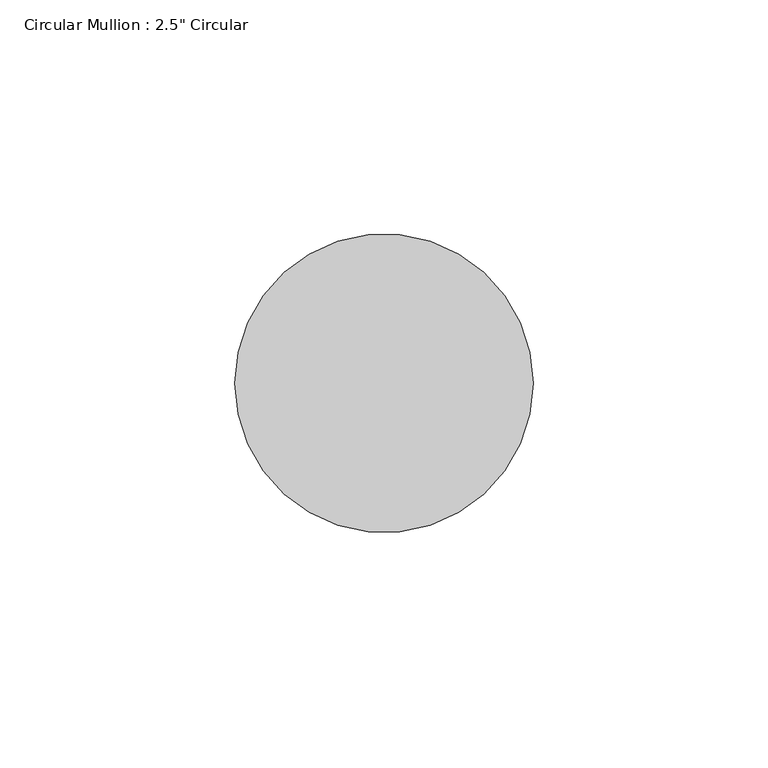
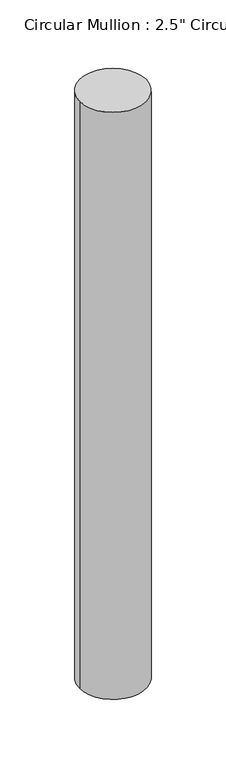
"""IFC4 building model written with IfcOpenShell, lengths in millimetres: member geometry."""

from ifc_helpers import new_model, si_unit, point, frame, origin, origin_2d, place, context, project, spatial, circle_curve, trimmed, segment, composite_curve, outline, extrude, source, transform, mapped, element, save


def member_1c8f807b(model_context):
    return source(origin(), model_context, "Body", "SweptSolid", [
        extrude(outline(composite_curve([segment(trimmed(circle_curve(origin_2d(), 31.75), [point((31.75, 0.0))], [point((-31.75, 0.0))], False, "CARTESIAN"), True, "CONTINUOUS"), segment(trimmed(circle_curve(origin_2d(), 31.75), [point((-31.75, 0.0))], [point((31.75, 0.0))], False, "CARTESIAN"), True, "CONTINUOUS")], self_intersect=False)), frame((0.0, 0.0, -592.6666667), z_axis=(0.0, 0.0, 1.0), x_axis=(1.0, 0.0, 0.0)), (0.0, 0.0, 1.0), 592.6666667),
    ])


if __name__ == "__main__":
    model = new_model("IFC4")
    model_context = context("Model", 3, world=origin())
    ifc_project = project(units=[si_unit("LENGTHUNIT", "METRE", prefix="MILLI")], contexts=[model_context])
    site = spatial("IfcSite", under=ifc_project)
    building = spatial("IfcBuilding", under=site)
    placement = place(None, origin())
    member_shape = member_1c8f807b(model_context)
    element("IfcMember", 1, ObjectType="Circular Mullion : 2.5\" Circular", at=placement, inside=building, context=model_context, shape_type="MappedRepresentation", body=[
        mapped(member_shape, transform((0.0, 0.0, 0.0), x_axis=(1.0, 0.0, 0.0), y_axis=(0.0, 1.0, 0.0), z_axis=(0.0, 0.0, 1.0))),
    ])
    save(model, "model.ifc")

# Revit data of these elements
# Type "Circular Mullion : 2.5\" Circular"
#   built-in parameter 1007350 = 0.104167 (stored number, unit not read)
# Element 1 (IfcMember, "Circular Mullion : 2.5\" Circular")
#   Materials on its faces: "Door - Frame"
# Materials
#   "Door - Frame": colour RGB 118 70 51, transparency 0, Cost = 0
